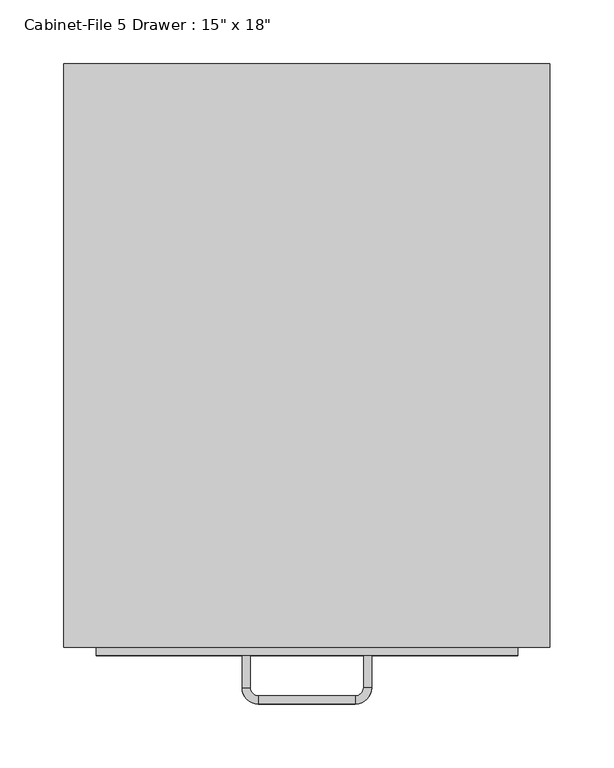
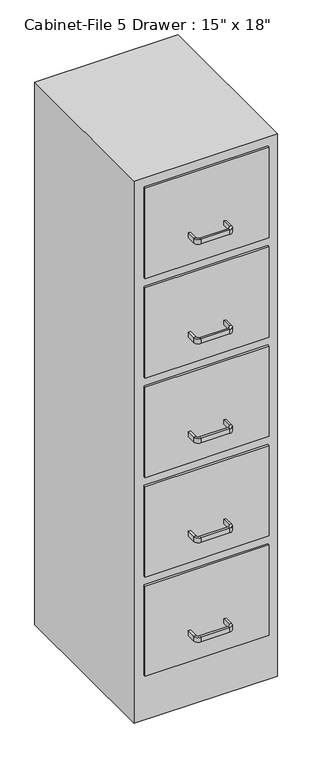
"""IFC4 building model written with IfcOpenShell, lengths in millimetres: furniture geometry."""

from ifc_helpers import new_model, si_unit, frame, origin, origin_with_axes, place, context, project, spatial, polyline, circle_curve, outline, extrude, source, transform, mapped, element, save
from ifc_brep_helpers import plane_surface, cylinder_surface, revolved_surface, advanced_brep


def furniture_d4d3357e(model_context):
    return source(origin(), model_context, "Body", "SolidModel", [
        extrude(outline(polyline([(62.603553, 86.4656999), (62.603553, -370.7343001), (-318.396447, -370.7343001), (-318.396447, 86.4656999), (62.603553, 86.4656999)])), origin_with_axes(), (0.0, 0.0, 1.0), 1524.0),
        extrude(outline(polyline([(37.203553, -377.0843001), (-292.996447, -377.0843001), (-292.996447, -370.7343001), (37.203553, -370.7343001), (37.203553, -377.0843001)])), frame((0.0, 0.0, 1244.6), z_axis=(0.0, 0.0, 1.0), x_axis=(1.0, 0.0, 0.0)), (0.0, 0.0, 1.0), 254.0),
        extrude(outline(polyline([(37.203553, -377.0843001), (-292.996447, -377.0843001), (-292.996447, -370.7343001), (37.203553, -370.7343001), (37.203553, -377.0843001)])), frame((0.0, 0.0, 965.2), z_axis=(0.0, 0.0, 1.0), x_axis=(1.0, 0.0, 0.0)), (0.0, 0.0, 1.0), 254.0),
        extrude(outline(polyline([(37.203553, -377.0843001), (-292.996447, -377.0843001), (-292.996447, -370.7343001), (37.203553, -370.7343001), (37.203553, -377.0843001)])), frame((0.0, 0.0, 685.8), z_axis=(0.0, 0.0, 1.0), x_axis=(1.0, 0.0, 0.0)), (0.0, 0.0, 1.0), 254.0),
        extrude(outline(polyline([(37.203553, -377.0843001), (-292.996447, -377.0843001), (-292.996447, -370.7343001), (37.203553, -370.7343001), (37.203553, -377.0843001)])), frame((0.0, 0.0, 406.4), z_axis=(0.0, 0.0, 1.0), x_axis=(1.0, 0.0, 0.0)), (0.0, 0.0, 1.0), 254.0),
        extrude(outline(polyline([(37.203553, -377.0843001), (-292.996447, -377.0843001), (-292.996447, -370.7343001), (37.203553, -370.7343001), (37.203553, -377.0843001)])), frame((0.0, 0.0, 127.0), z_axis=(0.0, 0.0, 1.0), x_axis=(1.0, 0.0, 0.0)), (0.0, 0.0, 1.0), 254.0),
        advanced_brep(
        [(-172.346447, -377.0843001, 203.2), (-178.696447, -377.0843001, 203.2), (-178.696447, -377.0843001, 215.9), (-172.346447, -377.0843001, 215.9), (-172.346447, -402.4843001, 203.2), (-178.696447, -402.4843001, 203.2), (-178.696447, -402.4843001, 215.9), (-172.346447, -402.4843001, 215.9), (-165.996447, -415.1843001, 203.2), (-165.996447, -408.8343001, 203.2), (-165.996447, -415.1843001, 215.9), (-165.996447, -408.8343001, 215.9), (-89.796447, -408.8343001, 203.2), (-89.796447, -415.1843001, 203.2), (-89.796447, -415.1843001, 215.9), (-89.796447, -408.8343001, 215.9), (-77.096447, -402.4843001, 203.2), (-83.446447, -402.4843001, 203.2), (-77.096447, -402.4843001, 215.9), (-83.446447, -402.4843001, 215.9), (-83.446447, -377.0843001, 203.2), (-83.446447, -377.0843001, 215.9), (-77.096447, -377.0843001, 215.9), (-77.096447, -377.0843001, 203.2)],
        [
            (0, 1),
            (1, 2),
            (2, 3),
            (3, 0),
            (0, 4),
            (4, 5),
            (5, 1),
            (5, 6),
            (6, 2),
            (6, 7),
            (7, 3),
            (7, 4),
            (8, 5, circle_curve(frame((-165.996447, -402.4843001, 203.2), z_axis=(0.0, 0.0, -1.0), x_axis=(-1.0, 0.0, 0.0)), 12.7)),
            (4, 9, circle_curve(frame((-165.996447, -402.4843001, 203.2), z_axis=(0.0, 0.0, 1.0), x_axis=(-1.0, 0.0, 0.0)), 6.35)),
            (9, 8),
            (10, 6, circle_curve(frame((-165.996447, -402.4843001, 215.9), z_axis=(0.0, 0.0, -1.0), x_axis=(-1.0, 0.0, 0.0)), 12.7)),
            (8, 10),
            (11, 7, circle_curve(frame((-165.996447, -402.4843001, 215.9), z_axis=(0.0, 0.0, -1.0), x_axis=(-1.0, 0.0, 0.0)), 6.35)),
            (10, 11),
            (11, 9),
            (9, 12),
            (12, 13),
            (13, 8),
            (13, 14),
            (14, 10),
            (14, 15),
            (15, 11),
            (15, 12),
            (16, 13, circle_curve(frame((-89.796447, -402.4843001, 203.2), z_axis=(0.0, 0.0, -1.0), x_axis=(0.0, -1.0, 0.0)), 12.7)),
            (12, 17, circle_curve(frame((-89.796447, -402.4843001, 203.2), z_axis=(0.0, 0.0, 1.0), x_axis=(0.0, -1.0, 0.0)), 6.35)),
            (17, 16),
            (18, 14, circle_curve(frame((-89.796447, -402.4843001, 215.9), z_axis=(0.0, 0.0, -1.0), x_axis=(0.0, -1.0, 0.0)), 12.7)),
            (16, 18),
            (19, 15, circle_curve(frame((-89.796447, -402.4843001, 215.9), z_axis=(0.0, 0.0, -1.0), x_axis=(0.0, -1.0, 0.0)), 6.35)),
            (18, 19),
            (19, 17),
            (20, 21),
            (21, 22),
            (22, 23),
            (23, 20),
            (17, 20),
            (23, 16),
            (22, 18),
            (21, 19),
        ],
        [
            plane_surface(frame((-1512.211566, -377.0843001, 0.0), z_axis=(0.0, 1.0, 0.0), x_axis=(0.0, 0.0, -1.0))),
            plane_surface(frame((-172.346447, -377.0843001, 203.2), z_axis=(0.0, 0.0, -1.0), x_axis=(0.0, -1.0, 0.0))),
            plane_surface(frame((-178.696447, -377.0843001, 203.2), z_axis=(-1.0, 0.0, 0.0), x_axis=(0.0, -1.0, 0.0))),
            plane_surface(frame((-178.696447, -377.0843001, 215.9), z_axis=(0.0, 0.0, 1.0), x_axis=(0.0, -1.0, 0.0))),
            plane_surface(frame((-172.346447, -377.0843001, 215.9), z_axis=(1.0, 0.0, 0.0), x_axis=(0.0, -1.0, 0.0))),
            plane_surface(frame((-165.996447, -402.4843001, 203.2), z_axis=(0.0, 0.0, -1.0), x_axis=(-1.0, 0.0, 0.0))),
            cylinder_surface(frame((-165.996447, -402.4843001, 0.0), z_axis=(0.0, 0.0, 1.0), x_axis=(-1.0, 0.0, 0.0)), 12.7),
            plane_surface(frame((-165.996447, -402.4843001, 215.9), z_axis=(0.0, 0.0, 1.0), x_axis=(-1.0, 0.0, 0.0))),
            revolved_surface(polyline([(-172.34644699999998, -402.4843001, 215.9), (-172.34644699999998, -402.4843001, 203.2)]), (-165.996447, -402.4843001, 0.0), (0.0, 0.0, 1.0)),
            plane_surface(frame((-165.996447, -408.8343001, 203.2), z_axis=(0.0, 0.0, -1.0), x_axis=(1.0, 0.0, 0.0))),
            plane_surface(frame((-165.996447, -415.1843001, 203.2), z_axis=(0.0, -1.0, 0.0), x_axis=(1.0, 0.0, 0.0))),
            plane_surface(frame((-165.996447, -415.1843001, 215.9), z_axis=(0.0, 0.0, 1.0), x_axis=(1.0, 0.0, 0.0))),
            plane_surface(frame((-165.996447, -408.8343001, 215.9), z_axis=(0.0, 1.0, 0.0), x_axis=(1.0, 0.0, 0.0))),
            plane_surface(frame((-89.796447, -402.4843001, 203.2), z_axis=(0.0, 0.0, -1.0), x_axis=(0.0, -1.0, 0.0))),
            cylinder_surface(frame((-89.796447, -402.4843001, 0.0), z_axis=(0.0, 0.0, 1.0), x_axis=(0.0, -1.0, 0.0)), 12.7),
            plane_surface(frame((-89.796447, -402.4843001, 215.9), z_axis=(0.0, 0.0, 1.0), x_axis=(0.0, -1.0, 0.0))),
            revolved_surface(polyline([(-89.796447, -408.8343001, 215.9), (-89.796447, -408.8343001, 203.2)]), (-89.796447, -402.4843001, 0.0), (0.0, 0.0, 1.0)),
            plane_surface(frame((-1410.611566, -377.0843001, 0.0), z_axis=(0.0, 1.0, 0.0), x_axis=(0.0, 0.0, 1.0))),
            plane_surface(frame((-83.446447, -402.4843001, 203.2), z_axis=(0.0, 0.0, -1.0), x_axis=(0.0, 1.0, 0.0))),
            plane_surface(frame((-77.096447, -402.4843001, 203.2), z_axis=(1.0, 0.0, 0.0), x_axis=(0.0, 1.0, 0.0))),
            plane_surface(frame((-77.096447, -402.4843001, 215.9), z_axis=(0.0, 0.0, 1.0), x_axis=(0.0, 1.0, 0.0))),
            plane_surface(frame((-83.446447, -402.4843001, 215.9), z_axis=(-1.0, 0.0, 0.0), x_axis=(0.0, 1.0, 0.0))),
        ],
        [
            (0, [[1, 2, 3, 4]]),
            (1, [[-1, 5, 6, 7]]),
            (2, [[-2, -7, 8, 9]]),
            (3, [[-3, -9, 10, 11]]),
            (4, [[-4, -11, 12, -5]]),
            (5, [[13, -6, 14, 15]]),
            (6, [[16, -8, -13, 17]]),
            (7, [[18, -10, -16, 19]]),
            (8, [[-14, -12, -18, 20]]),
            (9, [[-15, 21, 22, 23]]),
            (10, [[-17, -23, 24, 25]]),
            (11, [[-19, -25, 26, 27]]),
            (12, [[-20, -27, 28, -21]]),
            (13, [[29, -22, 30, 31]]),
            (14, [[32, -24, -29, 33]]),
            (15, [[34, -26, -32, 35]]),
            (16, [[-30, -28, -34, 36]]),
            (17, [[37, 38, 39, 40]]),
            (18, [[-31, 41, -40, 42]]),
            (19, [[-33, -42, -39, 43]]),
            (20, [[-35, -43, -38, 44]]),
            (21, [[-36, -44, -37, -41]]),
        ],
    ),
        advanced_brep(
        [(-172.346447, -377.0843001, 482.6), (-178.696447, -377.0843001, 482.6), (-178.696447, -377.0843001, 495.3), (-172.346447, -377.0843001, 495.3), (-172.346447, -402.4843001, 482.6), (-178.696447, -402.4843001, 482.6), (-178.696447, -402.4843001, 495.3), (-172.346447, -402.4843001, 495.3), (-165.996447, -415.1843001, 482.6), (-165.996447, -408.8343001, 482.6), (-165.996447, -415.1843001, 495.3), (-165.996447, -408.8343001, 495.3), (-89.796447, -408.8343001, 482.6), (-89.796447, -415.1843001, 482.6), (-89.796447, -415.1843001, 495.3), (-89.796447, -408.8343001, 495.3), (-77.096447, -402.4843001, 482.6), (-83.446447, -402.4843001, 482.6), (-77.096447, -402.4843001, 495.3), (-83.446447, -402.4843001, 495.3), (-83.446447, -377.0843001, 482.6), (-83.446447, -377.0843001, 495.3), (-77.096447, -377.0843001, 495.3), (-77.096447, -377.0843001, 482.6)],
        [
            (0, 1),
            (1, 2),
            (2, 3),
            (3, 0),
            (0, 4),
            (4, 5),
            (5, 1),
            (5, 6),
            (6, 2),
            (6, 7),
            (7, 3),
            (7, 4),
            (8, 5, circle_curve(frame((-165.996447, -402.4843001, 482.6), z_axis=(0.0, 0.0, -1.0), x_axis=(-1.0, 0.0, 0.0)), 12.7)),
            (4, 9, circle_curve(frame((-165.996447, -402.4843001, 482.6), z_axis=(0.0, 0.0, 1.0), x_axis=(-1.0, 0.0, 0.0)), 6.35)),
            (9, 8),
            (10, 6, circle_curve(frame((-165.996447, -402.4843001, 495.3), z_axis=(0.0, 0.0, -1.0), x_axis=(-1.0, 0.0, 0.0)), 12.7)),
            (8, 10),
            (11, 7, circle_curve(frame((-165.996447, -402.4843001, 495.3), z_axis=(0.0, 0.0, -1.0), x_axis=(-1.0, 0.0, 0.0)), 6.35)),
            (10, 11),
            (11, 9),
            (9, 12),
            (12, 13),
            (13, 8),
            (13, 14),
            (14, 10),
            (14, 15),
            (15, 11),
            (15, 12),
            (16, 13, circle_curve(frame((-89.796447, -402.4843001, 482.6), z_axis=(0.0, 0.0, -1.0), x_axis=(0.0, -1.0, 0.0)), 12.7)),
            (12, 17, circle_curve(frame((-89.796447, -402.4843001, 482.6), z_axis=(0.0, 0.0, 1.0), x_axis=(0.0, -1.0, 0.0)), 6.35)),
            (17, 16),
            (18, 14, circle_curve(frame((-89.796447, -402.4843001, 495.3), z_axis=(0.0, 0.0, -1.0), x_axis=(0.0, -1.0, 0.0)), 12.7)),
            (16, 18),
            (19, 15, circle_curve(frame((-89.796447, -402.4843001, 495.3), z_axis=(0.0, 0.0, -1.0), x_axis=(0.0, -1.0, 0.0)), 6.35)),
            (18, 19),
            (19, 17),
            (20, 21),
            (21, 22),
            (22, 23),
            (23, 20),
            (17, 20),
            (23, 16),
            (22, 18),
            (21, 19),
        ],
        [
            plane_surface(frame((-1512.211566, -377.0843001, 0.0), z_axis=(0.0, 1.0, 0.0), x_axis=(0.0, 0.0, -1.0))),
            plane_surface(frame((-172.346447, -377.0843001, 482.6), z_axis=(0.0, 0.0, -1.0), x_axis=(0.0, -1.0, 0.0))),
            plane_surface(frame((-178.696447, -377.0843001, 482.6), z_axis=(-1.0, 0.0, 0.0), x_axis=(0.0, -1.0, 0.0))),
            plane_surface(frame((-178.696447, -377.0843001, 495.3), z_axis=(0.0, 0.0, 1.0), x_axis=(0.0, -1.0, 0.0))),
            plane_surface(frame((-172.346447, -377.0843001, 495.3), z_axis=(1.0, 0.0, 0.0), x_axis=(0.0, -1.0, 0.0))),
            plane_surface(frame((-165.996447, -402.4843001, 482.6), z_axis=(0.0, 0.0, -1.0), x_axis=(-1.0, 0.0, 0.0))),
            cylinder_surface(frame((-165.996447, -402.4843001, 0.0), z_axis=(0.0, 0.0, 1.0), x_axis=(-1.0, 0.0, 0.0)), 12.7),
            plane_surface(frame((-165.996447, -402.4843001, 495.3), z_axis=(0.0, 0.0, 1.0), x_axis=(-1.0, 0.0, 0.0))),
            revolved_surface(polyline([(-172.34644699999998, -402.4843001, 495.3), (-172.34644699999998, -402.4843001, 482.6)]), (-165.996447, -402.4843001, 0.0), (0.0, 0.0, 1.0)),
            plane_surface(frame((-165.996447, -408.8343001, 482.6), z_axis=(0.0, 0.0, -1.0), x_axis=(1.0, 0.0, 0.0))),
            plane_surface(frame((-165.996447, -415.1843001, 482.6), z_axis=(0.0, -1.0, 0.0), x_axis=(1.0, 0.0, 0.0))),
            plane_surface(frame((-165.996447, -415.1843001, 495.3), z_axis=(0.0, 0.0, 1.0), x_axis=(1.0, 0.0, 0.0))),
            plane_surface(frame((-165.996447, -408.8343001, 495.3), z_axis=(0.0, 1.0, 0.0), x_axis=(1.0, 0.0, 0.0))),
            plane_surface(frame((-89.796447, -402.4843001, 482.6), z_axis=(0.0, 0.0, -1.0), x_axis=(0.0, -1.0, 0.0))),
            cylinder_surface(frame((-89.796447, -402.4843001, 0.0), z_axis=(0.0, 0.0, 1.0), x_axis=(0.0, -1.0, 0.0)), 12.7),
            plane_surface(frame((-89.796447, -402.4843001, 495.3), z_axis=(0.0, 0.0, 1.0), x_axis=(0.0, -1.0, 0.0))),
            revolved_surface(polyline([(-89.796447, -408.8343001, 495.3), (-89.796447, -408.8343001, 482.6)]), (-89.796447, -402.4843001, 0.0), (0.0, 0.0, 1.0)),
            plane_surface(frame((-1410.611566, -377.0843001, 0.0), z_axis=(0.0, 1.0, 0.0), x_axis=(0.0, 0.0, 1.0))),
            plane_surface(frame((-83.446447, -402.4843001, 482.6), z_axis=(0.0, 0.0, -1.0), x_axis=(0.0, 1.0, 0.0))),
            plane_surface(frame((-77.096447, -402.4843001, 482.6), z_axis=(1.0, 0.0, 0.0), x_axis=(0.0, 1.0, 0.0))),
            plane_surface(frame((-77.096447, -402.4843001, 495.3), z_axis=(0.0, 0.0, 1.0), x_axis=(0.0, 1.0, 0.0))),
            plane_surface(frame((-83.446447, -402.4843001, 495.3), z_axis=(-1.0, 0.0, 0.0), x_axis=(0.0, 1.0, 0.0))),
        ],
        [
            (0, [[1, 2, 3, 4]]),
            (1, [[-1, 5, 6, 7]]),
            (2, [[-2, -7, 8, 9]]),
            (3, [[-3, -9, 10, 11]]),
            (4, [[-4, -11, 12, -5]]),
            (5, [[13, -6, 14, 15]]),
            (6, [[16, -8, -13, 17]]),
            (7, [[18, -10, -16, 19]]),
            (8, [[-14, -12, -18, 20]]),
            (9, [[-15, 21, 22, 23]]),
            (10, [[-17, -23, 24, 25]]),
            (11, [[-19, -25, 26, 27]]),
            (12, [[-20, -27, 28, -21]]),
            (13, [[29, -22, 30, 31]]),
            (14, [[32, -24, -29, 33]]),
            (15, [[34, -26, -32, 35]]),
            (16, [[-30, -28, -34, 36]]),
            (17, [[37, 38, 39, 40]]),
            (18, [[-31, 41, -40, 42]]),
            (19, [[-33, -42, -39, 43]]),
            (20, [[-35, -43, -38, 44]]),
            (21, [[-36, -44, -37, -41]]),
        ],
    ),
        advanced_brep(
        [(-172.346447, -377.0843001, 762.0), (-178.696447, -377.0843001, 762.0), (-178.696447, -377.0843001, 774.7), (-172.346447, -377.0843001, 774.7), (-172.346447, -402.4843001, 762.0), (-178.696447, -402.4843001, 762.0), (-178.696447, -402.4843001, 774.7), (-172.346447, -402.4843001, 774.7), (-165.996447, -415.1843001, 762.0), (-165.996447, -408.8343001, 762.0), (-165.996447, -415.1843001, 774.7), (-165.996447, -408.8343001, 774.7), (-89.796447, -408.8343001, 762.0), (-89.796447, -415.1843001, 762.0), (-89.796447, -415.1843001, 774.7), (-89.796447, -408.8343001, 774.7), (-77.096447, -402.4843001, 762.0), (-83.446447, -402.4843001, 762.0), (-77.096447, -402.4843001, 774.7), (-83.446447, -402.4843001, 774.7), (-83.446447, -377.0843001, 762.0), (-83.446447, -377.0843001, 774.7), (-77.096447, -377.0843001, 774.7), (-77.096447, -377.0843001, 762.0)],
        [
            (0, 1),
            (1, 2),
            (2, 3),
            (3, 0),
            (0, 4),
            (4, 5),
            (5, 1),
            (5, 6),
            (6, 2),
            (6, 7),
            (7, 3),
            (7, 4),
            (8, 5, circle_curve(frame((-165.996447, -402.4843001, 762.0), z_axis=(0.0, 0.0, -1.0), x_axis=(-1.0, 0.0, 0.0)), 12.7)),
            (4, 9, circle_curve(frame((-165.996447, -402.4843001, 762.0), z_axis=(0.0, 0.0, 1.0), x_axis=(-1.0, 0.0, 0.0)), 6.35)),
            (9, 8),
            (10, 6, circle_curve(frame((-165.996447, -402.4843001, 774.7), z_axis=(0.0, 0.0, -1.0), x_axis=(-1.0, 0.0, 0.0)), 12.7)),
            (8, 10),
            (11, 7, circle_curve(frame((-165.996447, -402.4843001, 774.7), z_axis=(0.0, 0.0, -1.0), x_axis=(-1.0, 0.0, 0.0)), 6.35)),
            (10, 11),
            (11, 9),
            (9, 12),
            (12, 13),
            (13, 8),
            (13, 14),
            (14, 10),
            (14, 15),
            (15, 11),
            (15, 12),
            (16, 13, circle_curve(frame((-89.796447, -402.4843001, 762.0), z_axis=(0.0, 0.0, -1.0), x_axis=(0.0, -1.0, 0.0)), 12.7)),
            (12, 17, circle_curve(frame((-89.796447, -402.4843001, 762.0), z_axis=(0.0, 0.0, 1.0), x_axis=(0.0, -1.0, 0.0)), 6.35)),
            (17, 16),
            (18, 14, circle_curve(frame((-89.796447, -402.4843001, 774.7), z_axis=(0.0, 0.0, -1.0), x_axis=(0.0, -1.0, 0.0)), 12.7)),
            (16, 18),
            (19, 15, circle_curve(frame((-89.796447, -402.4843001, 774.7), z_axis=(0.0, 0.0, -1.0), x_axis=(0.0, -1.0, 0.0)), 6.35)),
            (18, 19),
            (19, 17),
            (20, 21),
            (21, 22),
            (22, 23),
            (23, 20),
            (17, 20),
            (23, 16),
            (22, 18),
            (21, 19),
        ],
        [
            plane_surface(frame((-1512.211566, -377.0843001, 0.0), z_axis=(0.0, 1.0, 0.0), x_axis=(0.0, 0.0, -1.0))),
            plane_surface(frame((-172.346447, -377.0843001, 762.0), z_axis=(0.0, 0.0, -1.0), x_axis=(0.0, -1.0, 0.0))),
            plane_surface(frame((-178.696447, -377.0843001, 762.0), z_axis=(-1.0, 0.0, 0.0), x_axis=(0.0, -1.0, 0.0))),
            plane_surface(frame((-178.696447, -377.0843001, 774.7), z_axis=(0.0, 0.0, 1.0), x_axis=(0.0, -1.0, 0.0))),
            plane_surface(frame((-172.346447, -377.0843001, 774.7), z_axis=(1.0, 0.0, 0.0), x_axis=(0.0, -1.0, 0.0))),
            plane_surface(frame((-165.996447, -402.4843001, 762.0), z_axis=(0.0, 0.0, -1.0), x_axis=(-1.0, 0.0, 0.0))),
            cylinder_surface(frame((-165.996447, -402.4843001, 0.0), z_axis=(0.0, 0.0, 1.0), x_axis=(-1.0, 0.0, 0.0)), 12.7),
            plane_surface(frame((-165.996447, -402.4843001, 774.7), z_axis=(0.0, 0.0, 1.0), x_axis=(-1.0, 0.0, 0.0))),
            revolved_surface(polyline([(-172.34644699999998, -402.4843001, 774.7), (-172.34644699999998, -402.4843001, 762.0)]), (-165.996447, -402.4843001, 0.0), (0.0, 0.0, 1.0)),
            plane_surface(frame((-165.996447, -408.8343001, 762.0), z_axis=(0.0, 0.0, -1.0), x_axis=(1.0, 0.0, 0.0))),
            plane_surface(frame((-165.996447, -415.1843001, 762.0), z_axis=(0.0, -1.0, 0.0), x_axis=(1.0, 0.0, 0.0))),
            plane_surface(frame((-165.996447, -415.1843001, 774.7), z_axis=(0.0, 0.0, 1.0), x_axis=(1.0, 0.0, 0.0))),
            plane_surface(frame((-165.996447, -408.8343001, 774.7), z_axis=(0.0, 1.0, 0.0), x_axis=(1.0, 0.0, 0.0))),
            plane_surface(frame((-89.796447, -402.4843001, 762.0), z_axis=(0.0, 0.0, -1.0), x_axis=(0.0, -1.0, 0.0))),
            cylinder_surface(frame((-89.796447, -402.4843001, 0.0), z_axis=(0.0, 0.0, 1.0), x_axis=(0.0, -1.0, 0.0)), 12.7),
            plane_surface(frame((-89.796447, -402.4843001, 774.7), z_axis=(0.0, 0.0, 1.0), x_axis=(0.0, -1.0, 0.0))),
            revolved_surface(polyline([(-89.796447, -408.8343001, 774.7), (-89.796447, -408.8343001, 762.0)]), (-89.796447, -402.4843001, 0.0), (0.0, 0.0, 1.0)),
            plane_surface(frame((-1410.611566, -377.0843001, 0.0), z_axis=(0.0, 1.0, 0.0), x_axis=(0.0, 0.0, 1.0))),
            plane_surface(frame((-83.446447, -402.4843001, 762.0), z_axis=(0.0, 0.0, -1.0), x_axis=(0.0, 1.0, 0.0))),
            plane_surface(frame((-77.096447, -402.4843001, 762.0), z_axis=(1.0, 0.0, 0.0), x_axis=(0.0, 1.0, 0.0))),
            plane_surface(frame((-77.096447, -402.4843001, 774.7), z_axis=(0.0, 0.0, 1.0), x_axis=(0.0, 1.0, 0.0))),
            plane_surface(frame((-83.446447, -402.4843001, 774.7), z_axis=(-1.0, 0.0, 0.0), x_axis=(0.0, 1.0, 0.0))),
        ],
        [
            (0, [[1, 2, 3, 4]]),
            (1, [[-1, 5, 6, 7]]),
            (2, [[-2, -7, 8, 9]]),
            (3, [[-3, -9, 10, 11]]),
            (4, [[-4, -11, 12, -5]]),
            (5, [[13, -6, 14, 15]]),
            (6, [[16, -8, -13, 17]]),
            (7, [[18, -10, -16, 19]]),
            (8, [[-14, -12, -18, 20]]),
            (9, [[-15, 21, 22, 23]]),
            (10, [[-17, -23, 24, 25]]),
            (11, [[-19, -25, 26, 27]]),
            (12, [[-20, -27, 28, -21]]),
            (13, [[29, -22, 30, 31]]),
            (14, [[32, -24, -29, 33]]),
            (15, [[34, -26, -32, 35]]),
            (16, [[-30, -28, -34, 36]]),
            (17, [[37, 38, 39, 40]]),
            (18, [[-31, 41, -40, 42]]),
            (19, [[-33, -42, -39, 43]]),
            (20, [[-35, -43, -38, 44]]),
            (21, [[-36, -44, -37, -41]]),
        ],
    ),
        advanced_brep(
        [(-172.346447, -377.0843001, 1041.4), (-178.696447, -377.0843001, 1041.4), (-178.696447, -377.0843001, 1054.1), (-172.346447, -377.0843001, 1054.1), (-172.346447, -402.4843001, 1041.4), (-178.696447, -402.4843001, 1041.4), (-178.696447, -402.4843001, 1054.1), (-172.346447, -402.4843001, 1054.1), (-165.996447, -415.1843001, 1041.4), (-165.996447, -408.8343001, 1041.4), (-165.996447, -415.1843001, 1054.1), (-165.996447, -408.8343001, 1054.1), (-89.796447, -408.8343001, 1041.4), (-89.796447, -415.1843001, 1041.4), (-89.796447, -415.1843001, 1054.1), (-89.796447, -408.8343001, 1054.1), (-77.096447, -402.4843001, 1041.4), (-83.446447, -402.4843001, 1041.4), (-77.096447, -402.4843001, 1054.1), (-83.446447, -402.4843001, 1054.1), (-83.446447, -377.0843001, 1041.4), (-83.446447, -377.0843001, 1054.1), (-77.096447, -377.0843001, 1054.1), (-77.096447, -377.0843001, 1041.4)],
        [
            (0, 1),
            (1, 2),
            (2, 3),
            (3, 0),
            (0, 4),
            (4, 5),
            (5, 1),
            (5, 6),
            (6, 2),
            (6, 7),
            (7, 3),
            (7, 4),
            (8, 5, circle_curve(frame((-165.996447, -402.4843001, 1041.4), z_axis=(0.0, 0.0, -1.0), x_axis=(-1.0, 0.0, 0.0)), 12.7)),
            (4, 9, circle_curve(frame((-165.996447, -402.4843001, 1041.4), z_axis=(0.0, 0.0, 1.0), x_axis=(-1.0, 0.0, 0.0)), 6.35)),
            (9, 8),
            (10, 6, circle_curve(frame((-165.996447, -402.4843001, 1054.1), z_axis=(0.0, 0.0, -1.0), x_axis=(-1.0, 0.0, 0.0)), 12.7)),
            (8, 10),
            (11, 7, circle_curve(frame((-165.996447, -402.4843001, 1054.1), z_axis=(0.0, 0.0, -1.0), x_axis=(-1.0, 0.0, 0.0)), 6.35)),
            (10, 11),
            (11, 9),
            (9, 12),
            (12, 13),
            (13, 8),
            (13, 14),
            (14, 10),
            (14, 15),
            (15, 11),
            (15, 12),
            (16, 13, circle_curve(frame((-89.796447, -402.4843001, 1041.4), z_axis=(0.0, 0.0, -1.0), x_axis=(0.0, -1.0, 0.0)), 12.7)),
            (12, 17, circle_curve(frame((-89.796447, -402.4843001, 1041.4), z_axis=(0.0, 0.0, 1.0), x_axis=(0.0, -1.0, 0.0)), 6.35)),
            (17, 16),
            (18, 14, circle_curve(frame((-89.796447, -402.4843001, 1054.1), z_axis=(0.0, 0.0, -1.0), x_axis=(0.0, -1.0, 0.0)), 12.7)),
            (16, 18),
            (19, 15, circle_curve(frame((-89.796447, -402.4843001, 1054.1), z_axis=(0.0, 0.0, -1.0), x_axis=(0.0, -1.0, 0.0)), 6.35)),
            (18, 19),
            (19, 17),
            (20, 21),
            (21, 22),
            (22, 23),
            (23, 20),
            (17, 20),
            (23, 16),
            (22, 18),
            (21, 19),
        ],
        [
            plane_surface(frame((-1512.211566, -377.0843001, 0.0), z_axis=(0.0, 1.0, 0.0), x_axis=(0.0, 0.0, -1.0))),
            plane_surface(frame((-172.346447, -377.0843001, 1041.4), z_axis=(0.0, 0.0, -1.0), x_axis=(0.0, -1.0, 0.0))),
            plane_surface(frame((-178.696447, -377.0843001, 1041.4), z_axis=(-1.0, 0.0, 0.0), x_axis=(0.0, -1.0, 0.0))),
            plane_surface(frame((-178.696447, -377.0843001, 1054.1), z_axis=(0.0, 0.0, 1.0), x_axis=(0.0, -1.0, 0.0))),
            plane_surface(frame((-172.346447, -377.0843001, 1054.1), z_axis=(1.0, 0.0, 0.0), x_axis=(0.0, -1.0, 0.0))),
            plane_surface(frame((-165.996447, -402.4843001, 1041.4), z_axis=(0.0, 0.0, -1.0), x_axis=(-1.0, 0.0, 0.0))),
            cylinder_surface(frame((-165.996447, -402.4843001, 0.0), z_axis=(0.0, 0.0, 1.0), x_axis=(-1.0, 0.0, 0.0)), 12.7),
            plane_surface(frame((-165.996447, -402.4843001, 1054.1), z_axis=(0.0, 0.0, 1.0), x_axis=(-1.0, 0.0, 0.0))),
            revolved_surface(polyline([(-172.34644699999998, -402.4843001, 1054.1), (-172.34644699999998, -402.4843001, 1041.4)]), (-165.996447, -402.4843001, 0.0), (0.0, 0.0, 1.0)),
            plane_surface(frame((-165.996447, -408.8343001, 1041.4), z_axis=(0.0, 0.0, -1.0), x_axis=(1.0, 0.0, 0.0))),
            plane_surface(frame((-165.996447, -415.1843001, 1041.4), z_axis=(0.0, -1.0, 0.0), x_axis=(1.0, 0.0, 0.0))),
            plane_surface(frame((-165.996447, -415.1843001, 1054.1), z_axis=(0.0, 0.0, 1.0), x_axis=(1.0, 0.0, 0.0))),
            plane_surface(frame((-165.996447, -408.8343001, 1054.1), z_axis=(0.0, 1.0, 0.0), x_axis=(1.0, 0.0, 0.0))),
            plane_surface(frame((-89.796447, -402.4843001, 1041.4), z_axis=(0.0, 0.0, -1.0), x_axis=(0.0, -1.0, 0.0))),
            cylinder_surface(frame((-89.796447, -402.4843001, 0.0), z_axis=(0.0, 0.0, 1.0), x_axis=(0.0, -1.0, 0.0)), 12.7),
            plane_surface(frame((-89.796447, -402.4843001, 1054.1), z_axis=(0.0, 0.0, 1.0), x_axis=(0.0, -1.0, 0.0))),
            revolved_surface(polyline([(-89.796447, -408.8343001, 1054.1), (-89.796447, -408.8343001, 1041.4)]), (-89.796447, -402.4843001, 0.0), (0.0, 0.0, 1.0)),
            plane_surface(frame((-1410.611566, -377.0843001, 0.0), z_axis=(0.0, 1.0, 0.0), x_axis=(0.0, 0.0, 1.0))),
            plane_surface(frame((-83.446447, -402.4843001, 1041.4), z_axis=(0.0, 0.0, -1.0), x_axis=(0.0, 1.0, 0.0))),
            plane_surface(frame((-77.096447, -402.4843001, 1041.4), z_axis=(1.0, 0.0, 0.0), x_axis=(0.0, 1.0, 0.0))),
            plane_surface(frame((-77.096447, -402.4843001, 1054.1), z_axis=(0.0, 0.0, 1.0), x_axis=(0.0, 1.0, 0.0))),
            plane_surface(frame((-83.446447, -402.4843001, 1054.1), z_axis=(-1.0, 0.0, 0.0), x_axis=(0.0, 1.0, 0.0))),
        ],
        [
            (0, [[1, 2, 3, 4]]),
            (1, [[-1, 5, 6, 7]]),
            (2, [[-2, -7, 8, 9]]),
            (3, [[-3, -9, 10, 11]]),
            (4, [[-4, -11, 12, -5]]),
            (5, [[13, -6, 14, 15]]),
            (6, [[16, -8, -13, 17]]),
            (7, [[18, -10, -16, 19]]),
            (8, [[-14, -12, -18, 20]]),
            (9, [[-15, 21, 22, 23]]),
            (10, [[-17, -23, 24, 25]]),
            (11, [[-19, -25, 26, 27]]),
            (12, [[-20, -27, 28, -21]]),
            (13, [[29, -22, 30, 31]]),
            (14, [[32, -24, -29, 33]]),
            (15, [[34, -26, -32, 35]]),
            (16, [[-30, -28, -34, 36]]),
            (17, [[37, 38, 39, 40]]),
            (18, [[-31, 41, -40, 42]]),
            (19, [[-33, -42, -39, 43]]),
            (20, [[-35, -43, -38, 44]]),
            (21, [[-36, -44, -37, -41]]),
        ],
    ),
        advanced_brep(
        [(-172.346447, -377.0843001, 1320.8), (-178.696447, -377.0843001, 1320.8), (-178.696447, -377.0843001, 1333.5), (-172.346447, -377.0843001, 1333.5), (-172.346447, -402.4843001, 1320.8), (-178.696447, -402.4843001, 1320.8), (-178.696447, -402.4843001, 1333.5), (-172.346447, -402.4843001, 1333.5), (-165.996447, -415.1843001, 1320.8), (-165.996447, -408.8343001, 1320.8), (-165.996447, -415.1843001, 1333.5), (-165.996447, -408.8343001, 1333.5), (-89.796447, -408.8343001, 1320.8), (-89.796447, -415.1843001, 1320.8), (-89.796447, -415.1843001, 1333.5), (-89.796447, -408.8343001, 1333.5), (-77.096447, -402.4843001, 1320.8), (-83.446447, -402.4843001, 1320.8), (-77.096447, -402.4843001, 1333.5), (-83.446447, -402.4843001, 1333.5), (-83.446447, -377.0843001, 1320.8), (-83.446447, -377.0843001, 1333.5), (-77.096447, -377.0843001, 1333.5), (-77.096447, -377.0843001, 1320.8)],
        [
            (0, 1),
            (1, 2),
            (2, 3),
            (3, 0),
            (0, 4),
            (4, 5),
            (5, 1),
            (5, 6),
            (6, 2),
            (6, 7),
            (7, 3),
            (7, 4),
            (8, 5, circle_curve(frame((-165.996447, -402.4843001, 1320.8), z_axis=(0.0, 0.0, -1.0), x_axis=(-1.0, 0.0, 0.0)), 12.7)),
            (4, 9, circle_curve(frame((-165.996447, -402.4843001, 1320.8), z_axis=(0.0, 0.0, 1.0), x_axis=(-1.0, 0.0, 0.0)), 6.35)),
            (9, 8),
            (10, 6, circle_curve(frame((-165.996447, -402.4843001, 1333.5), z_axis=(0.0, 0.0, -1.0), x_axis=(-1.0, 0.0, 0.0)), 12.7)),
            (8, 10),
            (11, 7, circle_curve(frame((-165.996447, -402.4843001, 1333.5), z_axis=(0.0, 0.0, -1.0), x_axis=(-1.0, 0.0, 0.0)), 6.35)),
            (10, 11),
            (11, 9),
            (9, 12),
            (12, 13),
            (13, 8),
            (13, 14),
            (14, 10),
            (14, 15),
            (15, 11),
            (15, 12),
            (16, 13, circle_curve(frame((-89.796447, -402.4843001, 1320.8), z_axis=(0.0, 0.0, -1.0), x_axis=(0.0, -1.0, 0.0)), 12.7)),
            (12, 17, circle_curve(frame((-89.796447, -402.4843001, 1320.8), z_axis=(0.0, 0.0, 1.0), x_axis=(0.0, -1.0, 0.0)), 6.35)),
            (17, 16),
            (18, 14, circle_curve(frame((-89.796447, -402.4843001, 1333.5), z_axis=(0.0, 0.0, -1.0), x_axis=(0.0, -1.0, 0.0)), 12.7)),
            (16, 18),
            (19, 15, circle_curve(frame((-89.796447, -402.4843001, 1333.5), z_axis=(0.0, 0.0, -1.0), x_axis=(0.0, -1.0, 0.0)), 6.35)),
            (18, 19),
            (19, 17),
            (20, 21),
            (21, 22),
            (22, 23),
            (23, 20),
            (17, 20),
            (23, 16),
            (22, 18),
            (21, 19),
        ],
        [
            plane_surface(frame((-1512.211566, -377.0843001, 0.0), z_axis=(0.0, 1.0, 0.0), x_axis=(0.0, 0.0, -1.0))),
            plane_surface(frame((-172.346447, -377.0843001, 1320.8), z_axis=(0.0, 0.0, -1.0), x_axis=(0.0, -1.0, 0.0))),
            plane_surface(frame((-178.696447, -377.0843001, 1320.8), z_axis=(-1.0, 0.0, 0.0), x_axis=(0.0, -1.0, 0.0))),
            plane_surface(frame((-178.696447, -377.0843001, 1333.5), z_axis=(0.0, 0.0, 1.0), x_axis=(0.0, -1.0, 0.0))),
            plane_surface(frame((-172.346447, -377.0843001, 1333.5), z_axis=(1.0, 0.0, 0.0), x_axis=(0.0, -1.0, 0.0))),
            plane_surface(frame((-165.996447, -402.4843001, 1320.8), z_axis=(0.0, 0.0, -1.0), x_axis=(-1.0, 0.0, 0.0))),
            cylinder_surface(frame((-165.996447, -402.4843001, 0.0), z_axis=(0.0, 0.0, 1.0), x_axis=(-1.0, 0.0, 0.0)), 12.7),
            plane_surface(frame((-165.996447, -402.4843001, 1333.5), z_axis=(0.0, 0.0, 1.0), x_axis=(-1.0, 0.0, 0.0))),
            revolved_surface(polyline([(-172.34644699999998, -402.4843001, 1333.5), (-172.34644699999998, -402.4843001, 1320.8)]), (-165.996447, -402.4843001, 0.0), (0.0, 0.0, 1.0)),
            plane_surface(frame((-165.996447, -408.8343001, 1320.8), z_axis=(0.0, 0.0, -1.0), x_axis=(1.0, 0.0, 0.0))),
            plane_surface(frame((-165.996447, -415.1843001, 1320.8), z_axis=(0.0, -1.0, 0.0), x_axis=(1.0, 0.0, 0.0))),
            plane_surface(frame((-165.996447, -415.1843001, 1333.5), z_axis=(0.0, 0.0, 1.0), x_axis=(1.0, 0.0, 0.0))),
            plane_surface(frame((-165.996447, -408.8343001, 1333.5), z_axis=(0.0, 1.0, 0.0), x_axis=(1.0, 0.0, 0.0))),
            plane_surface(frame((-89.796447, -402.4843001, 1320.8), z_axis=(0.0, 0.0, -1.0), x_axis=(0.0, -1.0, 0.0))),
            cylinder_surface(frame((-89.796447, -402.4843001, 0.0), z_axis=(0.0, 0.0, 1.0), x_axis=(0.0, -1.0, 0.0)), 12.7),
            plane_surface(frame((-89.796447, -402.4843001, 1333.5), z_axis=(0.0, 0.0, 1.0), x_axis=(0.0, -1.0, 0.0))),
            revolved_surface(polyline([(-89.796447, -408.8343001, 1333.5), (-89.796447, -408.8343001, 1320.8)]), (-89.796447, -402.4843001, 0.0), (0.0, 0.0, 1.0)),
            plane_surface(frame((-1410.611566, -377.0843001, 0.0), z_axis=(0.0, 1.0, 0.0), x_axis=(0.0, 0.0, 1.0))),
            plane_surface(frame((-83.446447, -402.4843001, 1320.8), z_axis=(0.0, 0.0, -1.0), x_axis=(0.0, 1.0, 0.0))),
            plane_surface(frame((-77.096447, -402.4843001, 1320.8), z_axis=(1.0, 0.0, 0.0), x_axis=(0.0, 1.0, 0.0))),
            plane_surface(frame((-77.096447, -402.4843001, 1333.5), z_axis=(0.0, 0.0, 1.0), x_axis=(0.0, 1.0, 0.0))),
            plane_surface(frame((-83.446447, -402.4843001, 1333.5), z_axis=(-1.0, 0.0, 0.0), x_axis=(0.0, 1.0, 0.0))),
        ],
        [
            (0, [[1, 2, 3, 4]]),
            (1, [[-1, 5, 6, 7]]),
            (2, [[-2, -7, 8, 9]]),
            (3, [[-3, -9, 10, 11]]),
            (4, [[-4, -11, 12, -5]]),
            (5, [[13, -6, 14, 15]]),
            (6, [[16, -8, -13, 17]]),
            (7, [[18, -10, -16, 19]]),
            (8, [[-14, -12, -18, 20]]),
            (9, [[-15, 21, 22, 23]]),
            (10, [[-17, -23, 24, 25]]),
            (11, [[-19, -25, 26, 27]]),
            (12, [[-20, -27, 28, -21]]),
            (13, [[29, -22, 30, 31]]),
            (14, [[32, -24, -29, 33]]),
            (15, [[34, -26, -32, 35]]),
            (16, [[-30, -28, -34, 36]]),
            (17, [[37, 38, 39, 40]]),
            (18, [[-31, 41, -40, 42]]),
            (19, [[-33, -42, -39, 43]]),
            (20, [[-35, -43, -38, 44]]),
            (21, [[-36, -44, -37, -41]]),
        ],
    ),
    ])


if __name__ == "__main__":
    model = new_model("IFC4")
    model_context = context("Model", 3, world=origin())
    ifc_project = project(units=[si_unit("LENGTHUNIT", "METRE", prefix="MILLI")], contexts=[model_context])
    site = spatial("IfcSite", under=ifc_project)
    building = spatial("IfcBuilding", under=site)
    placement = place(None, origin())
    furniture_shape = furniture_d4d3357e(model_context)
    element("IfcFurniture", 1, ObjectType="Cabinet-File 5 Drawer : 15\" x 18\"", at=placement, inside=building, context=model_context, shape_type="MappedRepresentation", body=[
        mapped(furniture_shape, transform((0.0, 0.0, 0.0), x_axis=(1.0, 0.0, 0.0), y_axis=(0.0, 1.0, 0.0), z_axis=(0.0, 0.0, 1.0))),
    ])
    save(model, "model.ifc")

# Revit data of these elements
# Type "Cabinet-File 5 Drawer : 15\" x 18\""
#   Assembly Code = "E2020200"
#   Depth = 1' - 6"
#   Height = 5' - 0"
#   Width = 1' - 3"
#   Cabinet Material = Steel, Paint Finish, Ivory, Glossy
#   Handle Material = Steel, Chrome Plated
#   Default Elevation = 0
# Element 1 (IfcFurniture, "Cabinet-File 5 Drawer : 15\" x 18\"")
#   Materials on its faces: "Steel, Chrome Plated", "Steel, Paint Finish, Ivory, Glossy"
# Materials
#   "Steel, Paint Finish, Ivory, Glossy": class "Metal", colour RGB 247 247 239, transparency 0, Description = "Steel, paint finish, ivory, glossy", Cost = 0
#   "Steel, Chrome Plated": class "Metal", colour RGB 17 17 17, transparency 0, Description = "Chromiuim plated steel", Cost = 0
